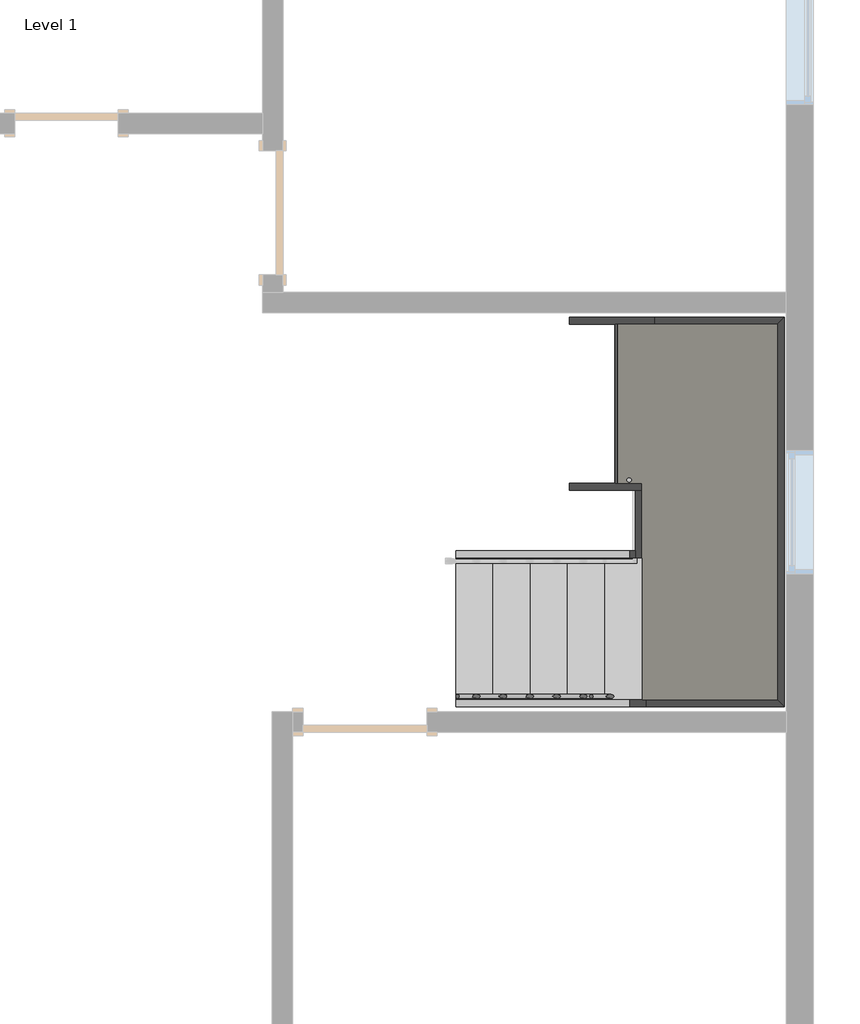
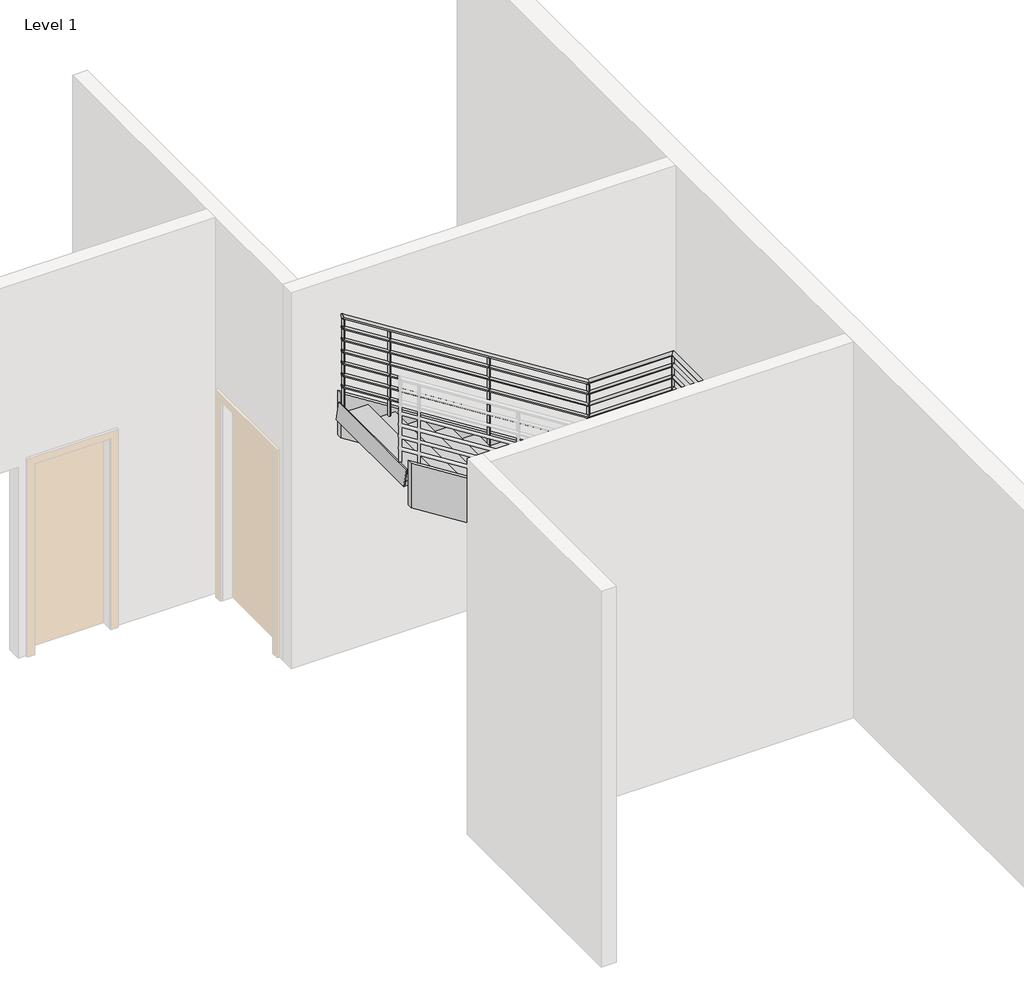
# One storey, part 3 of 3: 8 members, 2 stair flights, 1 railing, 1 slab.
"""IFC4 building model written with IfcOpenShell, lengths in millimetres."""

from ifc_helpers import new_model, si_unit, point, frame, frame_2d, origin, place, context, project, spatial, polyline, circle_curve, ellipse_curve, trimmed, segment, composite_curve, outline, extrude, faceted_brep, transform, mapped, element, save
from ifc_brep_helpers import plane_surface, cylinder_surface, advanced_brep
from components import non_monolithic_landing_709e637c, stair_flight_50mm_tread_25mm_nosing_13mm_riser_430ad9a4, stair_flight_50mm_tread_25mm_nosing_13mm_riser_1a1c1790

model = new_model("IFC4")

# Units and contexts
model_context = context("Model", 3, world=origin())
ifc_project = project(units=[si_unit("LENGTHUNIT", "METRE", prefix="MILLI")], contexts=[model_context])

# Site, building, storey
site = spatial("IfcSite", under=ifc_project)
building = spatial("IfcBuilding", under=site)
storey = spatial("IfcBuildingStorey", under=building, Name="Level 1", Elevation=0.0)

# Members
placement = place(None, origin())
element("IfcMember", 1, ObjectType="Stringer - 50mm Width", at=placement, inside=storey, context=model_context, shape_type="SweptSolid", body=[
    extrude(outline(polyline([(389.0025785, -528.272677), (0.0, -528.272677), (0.0, -395.0139442), (753.6703666, 796.727323), (1226.9472425, 796.727323), (389.0025785, -528.272677)])), frame((0.0, 4121.4539608, 0.0), z_axis=(0.0, 1.0, 0.0), x_axis=(0.0, 0.0, 1.0)), (0.0, 0.0, 1.0), 50.0),
])
element("IfcMember", 2, ObjectType="Stringer - 50mm Width", at=placement, inside=storey, context=model_context, shape_type="SweptSolid", body=[
    extrude(outline(polyline([(389.0025785, -528.272677), (0.0, -528.272677), (0.0, -395.0139442), (864.7850313, 972.4273866), (1264.7850313, 856.5583266), (389.0025785, -528.272677)])), frame((0.0, 3021.4281795, 0.0), z_axis=(0.0, 1.0, 0.0), x_axis=(0.0, 0.0, 1.0)), (0.0, 0.0, 1.0), 50.0),
])
element("IfcMember", 3, ObjectType="Stringer - 50mm Width", at=placement, inside=storey, context=model_context, shape_type="SweptSolid", body=[
    extrude(outline(polyline([(864.7850313, 846.727323), (1334.7593813, 846.727323), (2823.7851872, -1507.7947325), (2350.5083113, -1507.7947325), (864.7850313, 841.5052039), (864.7850313, 846.727323)])), frame((0.0, 4618.9227481, 0.0), z_axis=(0.0, 1.0, 0.0), x_axis=(0.0, 0.0, 1.0)), (0.0, 0.0, 1.0), 50.0),
])
element("IfcMember", 4, ObjectType="Stringer - 50mm Width", at=placement, inside=storey, context=model_context, shape_type="SweptSolid", body=[
    extrude(outline(polyline([(864.7850313, 841.5052039), (1264.7850313, 957.3742639), (2823.7851872, -1507.7947325), (2350.5083113, -1507.7947325), (864.7850313, 841.5052039)])), frame((0.0, 5845.1517528, 0.0), z_axis=(0.0, 1.0, 0.0), x_axis=(0.0, 0.0, 1.0)), (0.0, 0.0, 1.0), 50.0),
])
element("IfcMember", 5, ObjectType="Stringer - 50mm Width", at=placement, inside=storey, context=model_context, shape_type="SweptSolid", body=[
    extrude(outline(polyline([(796.727323, 4618.9227481), (846.727323, 4618.9227481), (846.727323, 4121.4539608), (796.727323, 4121.4539608), (796.727323, 4618.9227481)])), frame((0.0, 0.0, 864.7850313), z_axis=(0.0, 0.0, 1.0), x_axis=(1.0, 0.0, 0.0)), (0.0, 0.0, 1.0), 400.0),
])
element("IfcMember", 6, ObjectType="Stringer - 50mm Width", at=placement, inside=storey, context=model_context, shape_type="Brep", body=[
    faceted_brep([(856.5583266, 3071.4281795, 1264.7850313), (856.5583266, 3021.4281795, 1264.7850313), (1896.7531043, 3021.4281795, 1264.7850313), (1846.7531043, 3071.4281795, 1264.7850313), (972.4273866, 3071.4281795, 864.7850313), (1846.7531043, 3071.4281795, 864.7850313), (972.4273866, 3021.4281795, 864.7850313), (1896.7531043, 3021.4281795, 864.7850313)], [[[0, 1, 2, 3]], [[4, 0, 3, 5]], [[6, 4, 5, 7]], [[1, 6, 7, 2]], [[1, 0, 4, 6]], [[2, 7, 5, 3]]]),
])
element("IfcMember", 7, ObjectType="Stringer - 50mm Width", at=placement, inside=storey, context=model_context, shape_type="SweptSolid", body=[
    extrude(outline(polyline([(1896.7531043, 3021.4281795), (1846.7531043, 3071.4281795), (1846.7531043, 5845.1517528), (1896.7531043, 5895.1517528), (1896.7531043, 3021.4281795)])), frame((0.0, 0.0, 864.7850313), z_axis=(0.0, 0.0, 1.0), x_axis=(1.0, 0.0, 0.0)), (0.0, 0.0, 1.0), 400.0),
])
element("IfcMember", 8, ObjectType="Stringer - 50mm Width", at=placement, inside=storey, context=model_context, shape_type="Brep", body=[
    faceted_brep([(1846.7531043, 5845.1517528, 1264.7850313), (1896.7531043, 5895.1517528, 1264.7850313), (957.3742639, 5895.1517528, 1264.7850313), (957.3742639, 5845.1517528, 1264.7850313), (1846.7531043, 5845.1517528, 864.7850313), (841.5052039, 5845.1517528, 864.7850313), (1896.7531043, 5895.1517528, 864.7850313), (841.5052039, 5895.1517528, 864.7850313)], [[[0, 1, 2, 3]], [[4, 0, 3, 5]], [[6, 4, 5, 7]], [[1, 6, 7, 2]], [[1, 0, 4, 6]], [[2, 7, 5, 3]]]),
])

# Railing
element("IfcRailing", 9, ObjectType="900mm Pipe", at=placement, inside=storey, context=model_context, shape_type="SolidModel", body=[
    advanced_brep(
    [(-528.272677, 3076.8281795, 1224.1622432), (-528.272677, 3116.8281795, 1224.1622432), (852.520776, 3076.8281795, 2097.3913043), (852.520776, 3116.8281795, 2097.3913043), (1841.3531043, 3076.8281795, 2097.3913043), (1801.3531043, 3116.8281795, 2097.3913043), (1841.3531043, 5839.7517528, 2097.3913043), (1801.3531043, 5799.7517528, 2097.3913043), (961.4118145, 5839.7517528, 2097.3913043), (961.4118145, 5799.7517528, 2097.3913043), (-1507.7947325, 5839.7517528, 3658.9448519), (-1507.7947325, 5799.7517528, 3658.9448519)],
    [
        (0, 1, ellipse_curve(frame((-528.272677, 3096.8281795, 1224.1622432), z_axis=(-1.0, 0.0, 0.0), x_axis=(0.0, 0.0, -1.0)), 23.6638438, 20.0)),
        (1, 0, ellipse_curve(frame((-528.272677, 3096.8281795, 1224.1622432), z_axis=(-1.0, 0.0, 0.0), x_axis=(0.0, 0.0, -1.0)), 23.6638438, 20.0)),
        (0, 2),
        (2, 3, ellipse_curve(frame((852.520776, 3096.8281795, 2097.3913043), z_axis=(-0.9605132043335073, 0.0, -0.2782344053149755), x_axis=(0.27823440531497556, 0.0, -0.9605132043335073)), 20.822202, 20.0)),
        (3, 1),
        (3, 2, ellipse_curve(frame((852.520776, 3096.8281795, 2097.3913043), z_axis=(-0.9605132043335073, 0.0, -0.2782344053149755), x_axis=(0.27823440531497556, 0.0, -0.9605132043335073)), 20.822202, 20.0)),
        (2, 4),
        (4, 5, ellipse_curve(frame((1821.3531043, 3096.8281795, 2097.3913043), z_axis=(-0.7071067811865501, -0.7071067811865449, 0.0), x_axis=(-0.7071067811865449, 0.7071067811865501, 0.0)), 28.2842712, 20.0)),
        (5, 3),
        (5, 4, ellipse_curve(frame((1821.3531043, 3096.8281795, 2097.3913043), z_axis=(-0.7071067811865501, -0.7071067811865449, 0.0), x_axis=(-0.7071067811865449, 0.7071067811865501, 0.0)), 28.2842712, 20.0)),
        (4, 6),
        (6, 7, ellipse_curve(frame((1821.3531043, 5819.7517528, 2097.3913043), z_axis=(0.7071067811865449, -0.7071067811865501, 0.0), x_axis=(-0.70710678118655, -0.707106781186545, 0.0)), 28.2842712, 20.0)),
        (7, 5),
        (7, 6, ellipse_curve(frame((1821.3531043, 5819.7517528, 2097.3913043), z_axis=(0.7071067811865449, -0.7071067811865501, 0.0), x_axis=(-0.70710678118655, -0.707106781186545, 0.0)), 28.2842712, 20.0)),
        (6, 8),
        (8, 9, ellipse_curve(frame((961.4118145, 5819.7517528, 2097.3913043), z_axis=(0.9605132043335073, 0.0, -0.2782344053149753), x_axis=(0.27823440531497584, 0.0, 0.9605132043335073)), 20.822202, 20.0)),
        (9, 7),
        (9, 8, ellipse_curve(frame((961.4118145, 5819.7517528, 2097.3913043), z_axis=(0.9605132043335073, 0.0, -0.2782344053149753), x_axis=(0.27823440531497584, 0.0, 0.9605132043335073)), 20.822202, 20.0)),
        (10, 11, ellipse_curve(frame((-1507.7947325, 5819.7517528, 3658.9448519), z_axis=(-1.0, 0.0, 0.0), x_axis=(0.0, 0.0, -1.0)), 23.6638438, 20.0)),
        (11, 10, ellipse_curve(frame((-1507.7947325, 5819.7517528, 3658.9448519), z_axis=(-1.0, 0.0, 0.0), x_axis=(0.0, 0.0, -1.0)), 23.6638438, 20.0)),
        (8, 10),
        (11, 9),
    ],
    [
        plane_surface(frame((-528.272677, 3096.8281795, 1247.826087), z_axis=(-1.0, 0.0, 0.0), x_axis=(0.0, 1.0, 0.0))),
        cylinder_surface(frame((-517.5827642, 3096.8281795, 1230.9226623), z_axis=(-0.8451712313980438, 0.0, -0.5344956404098301), x_axis=(0.0, 1.0, 0.0)), 20.0),
        cylinder_surface(frame((846.727323, 3096.8281795, 2097.3913043), z_axis=(-1.0, 0.0, 0.0), x_axis=(0.0, 1.0, 0.0)), 20.0),
        cylinder_surface(frame((1821.3531043, 3096.8281795, 2097.3913043), z_axis=(0.0, -1.0, 0.0), x_axis=(-1.0, 0.0, 0.0)), 20.0),
        cylinder_surface(frame((1821.3531043, 5819.7517528, 2097.3913043), z_axis=(1.0, 0.0, 0.0), x_axis=(0.0, -1.0, 0.0)), 20.0),
        plane_surface(frame((-1507.7947325, 5819.7517528, 3682.6086957), z_axis=(-1.0, 0.0, 0.0), x_axis=(0.0, -1.0, 0.0))),
        cylinder_surface(frame((956.5153547, 5819.7517528, 2100.4878797), z_axis=(0.8451712313980441, 0.0, -0.5344956404098297), x_axis=(0.0, -1.0, 0.0)), 20.0),
    ],
    [
        (0, [[1, 2]]),
        (1, [[-1, 3, 4, 5]]),
        (1, [[-2, -5, 6, -3]]),
        (2, [[-4, 7, 8, 9]]),
        (2, [[-6, -9, 10, -7]]),
        (3, [[-8, 11, 12, 13]]),
        (3, [[-10, -13, 14, -11]]),
        (4, [[-12, 15, 16, 17]]),
        (4, [[-14, -17, 18, -15]]),
        (5, [[19, 20]]),
        (6, [[-16, 21, -20, 22]]),
        (6, [[-18, -22, -19, -21]]),
    ],
),
    advanced_brep(
    [(-528.272677, 3111.8281795, 1105.0782041), (-528.272677, 3081.8281795, 1105.0782041), (851.0724128, 3111.8281795, 1977.3913043), (851.0724128, 3081.8281795, 1977.3913043), (1806.3531043, 3111.8281795, 1977.3913043), (1836.3531043, 3081.8281795, 1977.3913043), (1806.3531043, 5804.7517528, 1977.3913043), (1836.3531043, 5834.7517528, 1977.3913043), (962.8601777, 5804.7517528, 1977.3913043), (962.8601777, 5834.7517528, 1977.3913043), (-1507.7947325, 5804.7517528, 3539.8608128), (-1507.7947325, 5834.7517528, 3539.8608128)],
    [
        (0, 1, ellipse_curve(frame((-528.272677, 3096.8281795, 1105.0782041), z_axis=(-1.0, 0.0, 0.0), x_axis=(0.0, 0.0, -1.0)), 17.7478828, 15.0)),
        (1, 0, ellipse_curve(frame((-528.272677, 3096.8281795, 1105.0782041), z_axis=(-1.0, 0.0, 0.0), x_axis=(0.0, 0.0, -1.0)), 17.7478828, 15.0)),
        (0, 2),
        (2, 3, ellipse_curve(frame((851.0724128, 3096.8281795, 1977.3913043), z_axis=(-0.9605132043335072, 0.0, -0.2782344053149755), x_axis=(0.2782344053149752, 0.0, -0.9605132043335075)), 15.6166515, 15.0)),
        (3, 1),
        (3, 2, ellipse_curve(frame((851.0724128, 3096.8281795, 1977.3913043), z_axis=(-0.9605132043335072, 0.0, -0.2782344053149755), x_axis=(0.2782344053149752, 0.0, -0.9605132043335075)), 15.6166515, 15.0)),
        (2, 4),
        (4, 5, ellipse_curve(frame((1821.3531043, 3096.8281795, 1977.3913043), z_axis=(-0.7071067811865501, -0.7071067811865449, 0.0), x_axis=(-0.7071067811865449, 0.7071067811865501, 0.0)), 21.2132034, 15.0)),
        (5, 3),
        (5, 4, ellipse_curve(frame((1821.3531043, 3096.8281795, 1977.3913043), z_axis=(-0.7071067811865501, -0.7071067811865449, 0.0), x_axis=(-0.7071067811865449, 0.7071067811865501, 0.0)), 21.2132034, 15.0)),
        (4, 6),
        (6, 7, ellipse_curve(frame((1821.3531043, 5819.7517528, 1977.3913043), z_axis=(0.7071067811865449, -0.7071067811865501, 0.0), x_axis=(-0.70710678118655, -0.707106781186545, 0.0)), 21.2132034, 15.0)),
        (7, 5),
        (7, 6, ellipse_curve(frame((1821.3531043, 5819.7517528, 1977.3913043), z_axis=(0.7071067811865449, -0.7071067811865501, 0.0), x_axis=(-0.70710678118655, -0.707106781186545, 0.0)), 21.2132034, 15.0)),
        (6, 8),
        (8, 9, ellipse_curve(frame((962.8601777, 5819.7517528, 1977.3913043), z_axis=(0.9605132043335073, 0.0, -0.27823440531497523), x_axis=(0.2782344053149759, 0.0, 0.9605132043335072)), 15.6166515, 15.0)),
        (9, 7),
        (9, 8, ellipse_curve(frame((962.8601777, 5819.7517528, 1977.3913043), z_axis=(0.9605132043335073, 0.0, -0.27823440531497523), x_axis=(0.2782344053149759, 0.0, 0.9605132043335072)), 15.6166515, 15.0)),
        (10, 11, ellipse_curve(frame((-1507.7947325, 5819.7517528, 3539.8608128), z_axis=(-1.0, 0.0, 0.0), x_axis=(0.0, 0.0, -1.0)), 17.7478828, 15.0)),
        (11, 10, ellipse_curve(frame((-1507.7947325, 5819.7517528, 3539.8608128), z_axis=(-1.0, 0.0, 0.0), x_axis=(0.0, 0.0, -1.0)), 17.7478828, 15.0)),
        (8, 10),
        (11, 9),
    ],
    [
        plane_surface(frame((-528.272677, 3096.8281795, 1122.826087), z_axis=(-1.0, 0.0, 0.0), x_axis=(0.0, 1.0, 0.0))),
        cylinder_surface(frame((-520.2552424, 3096.8281795, 1110.1485185), z_axis=(-0.8451712313980437, 0.0, -0.5344956404098301), x_axis=(0.0, -1.0, 0.0)), 15.0),
        cylinder_surface(frame((846.727323, 3096.8281795, 1977.3913043), z_axis=(-1.0, 0.0, 0.0), x_axis=(0.0, -1.0, 0.0)), 15.0),
        cylinder_surface(frame((1821.3531043, 3096.8281795, 1977.3913043), z_axis=(0.0, -1.0, 0.0), x_axis=(1.0, 0.0, 0.0)), 15.0),
        cylinder_surface(frame((1821.3531043, 5819.7517528, 1977.3913043), z_axis=(1.0, 0.0, 0.0), x_axis=(0.0, 1.0, 0.0)), 15.0),
        plane_surface(frame((-1507.7947325, 5819.7517528, 3557.6086957), z_axis=(-1.0, 0.0, 0.0), x_axis=(0.0, -1.0, 0.0))),
        cylinder_surface(frame((959.1878329, 5819.7517528, 1979.7137359), z_axis=(0.8451712313980441, 0.0, -0.5344956404098296), x_axis=(0.0, 1.0, 0.0)), 15.0),
    ],
    [
        (0, [[1, 2]]),
        (1, [[-1, 3, 4, 5]]),
        (1, [[-2, -5, 6, -3]]),
        (2, [[-4, 7, 8, 9]]),
        (2, [[-6, -9, 10, -7]]),
        (3, [[-8, 11, 12, 13]]),
        (3, [[-10, -13, 14, -11]]),
        (4, [[-12, 15, 16, 17]]),
        (4, [[-14, -17, 18, -15]]),
        (5, [[19, 20]]),
        (6, [[-16, 21, -20, 22]]),
        (6, [[-18, -22, -19, -21]]),
    ],
),
    advanced_brep(
    [(-528.272677, 3111.8281795, 980.0782041), (-528.272677, 3081.8281795, 980.0782041), (851.0724128, 3111.8281795, 1852.3913043), (851.0724128, 3081.8281795, 1852.3913043), (1806.3531043, 3111.8281795, 1852.3913043), (1836.3531043, 3081.8281795, 1852.3913043), (1806.3531043, 5804.7517528, 1852.3913043), (1836.3531043, 5834.7517528, 1852.3913043), (962.8601777, 5804.7517528, 1852.3913043), (962.8601777, 5834.7517528, 1852.3913043), (-1507.7947325, 5804.7517528, 3414.8608128), (-1507.7947325, 5834.7517528, 3414.8608128)],
    [
        (0, 1, ellipse_curve(frame((-528.272677, 3096.8281795, 980.0782041), z_axis=(-1.0, 0.0, 0.0), x_axis=(0.0, 0.0, -1.0)), 17.7478828, 15.0)),
        (1, 0, ellipse_curve(frame((-528.272677, 3096.8281795, 980.0782041), z_axis=(-1.0, 0.0, 0.0), x_axis=(0.0, 0.0, -1.0)), 17.7478828, 15.0)),
        (0, 2),
        (2, 3, ellipse_curve(frame((851.0724128, 3096.8281795, 1852.3913043), z_axis=(-0.9605132043335072, 0.0, -0.2782344053149755), x_axis=(0.2782344053149752, 0.0, -0.9605132043335075)), 15.6166515, 15.0)),
        (3, 1),
        (3, 2, ellipse_curve(frame((851.0724128, 3096.8281795, 1852.3913043), z_axis=(-0.9605132043335072, 0.0, -0.2782344053149755), x_axis=(0.2782344053149752, 0.0, -0.9605132043335075)), 15.6166515, 15.0)),
        (2, 4),
        (4, 5, ellipse_curve(frame((1821.3531043, 3096.8281795, 1852.3913043), z_axis=(-0.7071067811865501, -0.7071067811865449, 0.0), x_axis=(-0.7071067811865449, 0.7071067811865501, 0.0)), 21.2132034, 15.0)),
        (5, 3),
        (5, 4, ellipse_curve(frame((1821.3531043, 3096.8281795, 1852.3913043), z_axis=(-0.7071067811865501, -0.7071067811865449, 0.0), x_axis=(-0.7071067811865449, 0.7071067811865501, 0.0)), 21.2132034, 15.0)),
        (4, 6),
        (6, 7, ellipse_curve(frame((1821.3531043, 5819.7517528, 1852.3913043), z_axis=(0.7071067811865449, -0.7071067811865501, 0.0), x_axis=(-0.70710678118655, -0.707106781186545, 0.0)), 21.2132034, 15.0)),
        (7, 5),
        (7, 6, ellipse_curve(frame((1821.3531043, 5819.7517528, 1852.3913043), z_axis=(0.7071067811865449, -0.7071067811865501, 0.0), x_axis=(-0.70710678118655, -0.707106781186545, 0.0)), 21.2132034, 15.0)),
        (6, 8),
        (8, 9, ellipse_curve(frame((962.8601777, 5819.7517528, 1852.3913043), z_axis=(0.9605132043335073, 0.0, -0.2782344053149753), x_axis=(0.27823440531497584, 0.0, 0.9605132043335073)), 15.6166515, 15.0)),
        (9, 7),
        (9, 8, ellipse_curve(frame((962.8601777, 5819.7517528, 1852.3913043), z_axis=(0.9605132043335073, 0.0, -0.2782344053149753), x_axis=(0.27823440531497584, 0.0, 0.9605132043335073)), 15.6166515, 15.0)),
        (10, 11, ellipse_curve(frame((-1507.7947325, 5819.7517528, 3414.8608128), z_axis=(-1.0, 0.0, 0.0), x_axis=(0.0, 0.0, -1.0)), 17.7478828, 15.0)),
        (11, 10, ellipse_curve(frame((-1507.7947325, 5819.7517528, 3414.8608128), z_axis=(-1.0, 0.0, 0.0), x_axis=(0.0, 0.0, -1.0)), 17.7478828, 15.0)),
        (8, 10),
        (11, 9),
    ],
    [
        plane_surface(frame((-528.272677, 3096.8281795, 997.826087), z_axis=(-1.0, 0.0, 0.0), x_axis=(0.0, 1.0, 0.0))),
        cylinder_surface(frame((-520.2552424, 3096.8281795, 985.1485185), z_axis=(-0.8451712313980437, 0.0, -0.5344956404098301), x_axis=(0.0, -1.0, 0.0)), 15.0),
        cylinder_surface(frame((846.727323, 3096.8281795, 1852.3913043), z_axis=(-1.0, 0.0, 0.0), x_axis=(0.0, -1.0, 0.0)), 15.0),
        cylinder_surface(frame((1821.3531043, 3096.8281795, 1852.3913043), z_axis=(0.0, -1.0, 0.0), x_axis=(1.0, 0.0, 0.0)), 15.0),
        cylinder_surface(frame((1821.3531043, 5819.7517528, 1852.3913043), z_axis=(1.0, 0.0, 0.0), x_axis=(0.0, 1.0, 0.0)), 15.0),
        plane_surface(frame((-1507.7947325, 5819.7517528, 3432.6086957), z_axis=(-1.0, 0.0, 0.0), x_axis=(0.0, -1.0, 0.0))),
        cylinder_surface(frame((959.1878329, 5819.7517528, 1854.7137359), z_axis=(0.8451712313980441, 0.0, -0.5344956404098297), x_axis=(0.0, 1.0, 0.0)), 15.0),
    ],
    [
        (0, [[1, 2]]),
        (1, [[-1, 3, 4, 5]]),
        (1, [[-2, -5, 6, -3]]),
        (2, [[-4, 7, 8, 9]]),
        (2, [[-6, -9, 10, -7]]),
        (3, [[-8, 11, 12, 13]]),
        (3, [[-10, -13, 14, -11]]),
        (4, [[-12, 15, 16, 17]]),
        (4, [[-14, -17, 18, -15]]),
        (5, [[19, 20]]),
        (6, [[-16, 21, -20, 22]]),
        (6, [[-18, -22, -19, -21]]),
    ],
),
    advanced_brep(
    [(-528.272677, 3111.8281795, 855.0782041), (-528.272677, 3081.8281795, 855.0782041), (851.0724128, 3111.8281795, 1727.3913043), (851.0724128, 3081.8281795, 1727.3913043), (1806.3531043, 3111.8281795, 1727.3913043), (1836.3531043, 3081.8281795, 1727.3913043), (1806.3531043, 5804.7517528, 1727.3913043), (1836.3531043, 5834.7517528, 1727.3913043), (962.8601777, 5804.7517528, 1727.3913043), (962.8601777, 5834.7517528, 1727.3913043), (-1507.7947325, 5804.7517528, 3289.8608128), (-1507.7947325, 5834.7517528, 3289.8608128)],
    [
        (0, 1, ellipse_curve(frame((-528.272677, 3096.8281795, 855.0782041), z_axis=(-1.0, 0.0, 0.0), x_axis=(0.0, 0.0, -1.0)), 17.7478828, 15.0)),
        (1, 0, ellipse_curve(frame((-528.272677, 3096.8281795, 855.0782041), z_axis=(-1.0, 0.0, 0.0), x_axis=(0.0, 0.0, -1.0)), 17.7478828, 15.0)),
        (0, 2),
        (2, 3, ellipse_curve(frame((851.0724128, 3096.8281795, 1727.3913043), z_axis=(-0.9605132043335072, 0.0, -0.2782344053149755), x_axis=(0.2782344053149752, 0.0, -0.9605132043335075)), 15.6166515, 15.0)),
        (3, 1),
        (3, 2, ellipse_curve(frame((851.0724128, 3096.8281795, 1727.3913043), z_axis=(-0.9605132043335072, 0.0, -0.2782344053149755), x_axis=(0.2782344053149752, 0.0, -0.9605132043335075)), 15.6166515, 15.0)),
        (2, 4),
        (4, 5, ellipse_curve(frame((1821.3531043, 3096.8281795, 1727.3913043), z_axis=(-0.7071067811865501, -0.7071067811865449, 0.0), x_axis=(-0.7071067811865449, 0.7071067811865501, 0.0)), 21.2132034, 15.0)),
        (5, 3),
        (5, 4, ellipse_curve(frame((1821.3531043, 3096.8281795, 1727.3913043), z_axis=(-0.7071067811865501, -0.7071067811865449, 0.0), x_axis=(-0.7071067811865449, 0.7071067811865501, 0.0)), 21.2132034, 15.0)),
        (4, 6),
        (6, 7, ellipse_curve(frame((1821.3531043, 5819.7517528, 1727.3913043), z_axis=(0.7071067811865449, -0.7071067811865501, 0.0), x_axis=(-0.70710678118655, -0.707106781186545, 0.0)), 21.2132034, 15.0)),
        (7, 5),
        (7, 6, ellipse_curve(frame((1821.3531043, 5819.7517528, 1727.3913043), z_axis=(0.7071067811865449, -0.7071067811865501, 0.0), x_axis=(-0.70710678118655, -0.707106781186545, 0.0)), 21.2132034, 15.0)),
        (6, 8),
        (8, 9, ellipse_curve(frame((962.8601777, 5819.7517528, 1727.3913043), z_axis=(0.9605132043335073, 0.0, -0.2782344053149753), x_axis=(0.27823440531497584, 0.0, 0.9605132043335073)), 15.6166515, 15.0)),
        (9, 7),
        (9, 8, ellipse_curve(frame((962.8601777, 5819.7517528, 1727.3913043), z_axis=(0.9605132043335073, 0.0, -0.2782344053149753), x_axis=(0.27823440531497584, 0.0, 0.9605132043335073)), 15.6166515, 15.0)),
        (10, 11, ellipse_curve(frame((-1507.7947325, 5819.7517528, 3289.8608128), z_axis=(-1.0, 0.0, 0.0), x_axis=(0.0, 0.0, -1.0)), 17.7478828, 15.0)),
        (11, 10, ellipse_curve(frame((-1507.7947325, 5819.7517528, 3289.8608128), z_axis=(-1.0, 0.0, 0.0), x_axis=(0.0, 0.0, -1.0)), 17.7478828, 15.0)),
        (8, 10),
        (11, 9),
    ],
    [
        plane_surface(frame((-528.272677, 3096.8281795, 872.826087), z_axis=(-1.0, 0.0, 0.0), x_axis=(0.0, 1.0, 0.0))),
        cylinder_surface(frame((-520.2552424, 3096.8281795, 860.1485185), z_axis=(-0.8451712313980437, 0.0, -0.5344956404098301), x_axis=(0.0, -1.0, 0.0)), 15.0),
        cylinder_surface(frame((846.727323, 3096.8281795, 1727.3913043), z_axis=(-1.0, 0.0, 0.0), x_axis=(0.0, -1.0, 0.0)), 15.0),
        cylinder_surface(frame((1821.3531043, 3096.8281795, 1727.3913043), z_axis=(0.0, -1.0, 0.0), x_axis=(1.0, 0.0, 0.0)), 15.0),
        cylinder_surface(frame((1821.3531043, 5819.7517528, 1727.3913043), z_axis=(1.0, 0.0, 0.0), x_axis=(0.0, 1.0, 0.0)), 15.0),
        plane_surface(frame((-1507.7947325, 5819.7517528, 3307.6086957), z_axis=(-1.0, 0.0, 0.0), x_axis=(0.0, -1.0, 0.0))),
        cylinder_surface(frame((959.1878329, 5819.7517528, 1729.7137359), z_axis=(0.8451712313980441, 0.0, -0.5344956404098297), x_axis=(0.0, 1.0, 0.0)), 15.0),
    ],
    [
        (0, [[1, 2]]),
        (1, [[-1, 3, 4, 5]]),
        (1, [[-2, -5, 6, -3]]),
        (2, [[-4, 7, 8, 9]]),
        (2, [[-6, -9, 10, -7]]),
        (3, [[-8, 11, 12, 13]]),
        (3, [[-10, -13, 14, -11]]),
        (4, [[-12, 15, 16, 17]]),
        (4, [[-14, -17, 18, -15]]),
        (5, [[19, 20]]),
        (6, [[-16, 21, -20, 22]]),
        (6, [[-18, -22, -19, -21]]),
    ],
),
    advanced_brep(
    [(-528.272677, 3111.8281795, 730.0782041), (-528.272677, 3081.8281795, 730.0782041), (851.0724128, 3111.8281795, 1602.3913043), (851.0724128, 3081.8281795, 1602.3913043), (1806.3531043, 3111.8281795, 1602.3913043), (1836.3531043, 3081.8281795, 1602.3913043), (1806.3531043, 5804.7517528, 1602.3913043), (1836.3531043, 5834.7517528, 1602.3913043), (962.8601777, 5804.7517528, 1602.3913043), (962.8601777, 5834.7517528, 1602.3913043), (-1507.7947325, 5804.7517528, 3164.8608128), (-1507.7947325, 5834.7517528, 3164.8608128)],
    [
        (0, 1, ellipse_curve(frame((-528.272677, 3096.8281795, 730.0782041), z_axis=(-1.0, 0.0, 0.0), x_axis=(0.0, 0.0, -1.0)), 17.7478828, 15.0)),
        (1, 0, ellipse_curve(frame((-528.272677, 3096.8281795, 730.0782041), z_axis=(-1.0, 0.0, 0.0), x_axis=(0.0, 0.0, -1.0)), 17.7478828, 15.0)),
        (0, 2),
        (2, 3, ellipse_curve(frame((851.0724128, 3096.8281795, 1602.3913043), z_axis=(-0.9605132043335072, 0.0, -0.2782344053149755), x_axis=(0.2782344053149752, 0.0, -0.9605132043335075)), 15.6166515, 15.0)),
        (3, 1),
        (3, 2, ellipse_curve(frame((851.0724128, 3096.8281795, 1602.3913043), z_axis=(-0.9605132043335072, 0.0, -0.2782344053149755), x_axis=(0.2782344053149752, 0.0, -0.9605132043335075)), 15.6166515, 15.0)),
        (2, 4),
        (4, 5, ellipse_curve(frame((1821.3531043, 3096.8281795, 1602.3913043), z_axis=(-0.7071067811865501, -0.7071067811865449, 0.0), x_axis=(-0.7071067811865449, 0.7071067811865501, 0.0)), 21.2132034, 15.0)),
        (5, 3),
        (5, 4, ellipse_curve(frame((1821.3531043, 3096.8281795, 1602.3913043), z_axis=(-0.7071067811865501, -0.7071067811865449, 0.0), x_axis=(-0.7071067811865449, 0.7071067811865501, 0.0)), 21.2132034, 15.0)),
        (4, 6),
        (6, 7, ellipse_curve(frame((1821.3531043, 5819.7517528, 1602.3913043), z_axis=(0.7071067811865449, -0.7071067811865501, 0.0), x_axis=(-0.70710678118655, -0.707106781186545, 0.0)), 21.2132034, 15.0)),
        (7, 5),
        (7, 6, ellipse_curve(frame((1821.3531043, 5819.7517528, 1602.3913043), z_axis=(0.7071067811865449, -0.7071067811865501, 0.0), x_axis=(-0.70710678118655, -0.707106781186545, 0.0)), 21.2132034, 15.0)),
        (6, 8),
        (8, 9, ellipse_curve(frame((962.8601777, 5819.7517528, 1602.3913043), z_axis=(0.9605132043335073, 0.0, -0.2782344053149753), x_axis=(0.27823440531497584, 0.0, 0.9605132043335073)), 15.6166515, 15.0)),
        (9, 7),
        (9, 8, ellipse_curve(frame((962.8601777, 5819.7517528, 1602.3913043), z_axis=(0.9605132043335073, 0.0, -0.2782344053149753), x_axis=(0.27823440531497584, 0.0, 0.9605132043335073)), 15.6166515, 15.0)),
        (10, 11, ellipse_curve(frame((-1507.7947325, 5819.7517528, 3164.8608128), z_axis=(-1.0, 0.0, 0.0), x_axis=(0.0, 0.0, -1.0)), 17.7478828, 15.0)),
        (11, 10, ellipse_curve(frame((-1507.7947325, 5819.7517528, 3164.8608128), z_axis=(-1.0, 0.0, 0.0), x_axis=(0.0, 0.0, -1.0)), 17.7478828, 15.0)),
        (8, 10),
        (11, 9),
    ],
    [
        plane_surface(frame((-528.272677, 3096.8281795, 747.826087), z_axis=(-1.0, 0.0, 0.0), x_axis=(0.0, 1.0, 0.0))),
        cylinder_surface(frame((-520.2552424, 3096.8281795, 735.1485185), z_axis=(-0.8451712313980437, 0.0, -0.5344956404098301), x_axis=(0.0, -1.0, 0.0)), 15.0),
        cylinder_surface(frame((846.727323, 3096.8281795, 1602.3913043), z_axis=(-1.0, 0.0, 0.0), x_axis=(0.0, -1.0, 0.0)), 15.0),
        cylinder_surface(frame((1821.3531043, 3096.8281795, 1602.3913043), z_axis=(0.0, -1.0, 0.0), x_axis=(1.0, 0.0, 0.0)), 15.0),
        cylinder_surface(frame((1821.3531043, 5819.7517528, 1602.3913043), z_axis=(1.0, 0.0, 0.0), x_axis=(0.0, 1.0, 0.0)), 15.0),
        plane_surface(frame((-1507.7947325, 5819.7517528, 3182.6086957), z_axis=(-1.0, 0.0, 0.0), x_axis=(0.0, -1.0, 0.0))),
        cylinder_surface(frame((959.1878329, 5819.7517528, 1604.7137359), z_axis=(0.8451712313980441, 0.0, -0.5344956404098297), x_axis=(0.0, 1.0, 0.0)), 15.0),
    ],
    [
        (0, [[1, 2]]),
        (1, [[-1, 3, 4, 5]]),
        (1, [[-2, -5, 6, -3]]),
        (2, [[-4, 7, 8, 9]]),
        (2, [[-6, -9, 10, -7]]),
        (3, [[-8, 11, 12, 13]]),
        (3, [[-10, -13, 14, -11]]),
        (4, [[-12, 15, 16, 17]]),
        (4, [[-14, -17, 18, -15]]),
        (5, [[19, 20]]),
        (6, [[-16, 21, -20, 22]]),
        (6, [[-18, -22, -19, -21]]),
    ],
),
    advanced_brep(
    [(-528.272677, 3111.8281795, 605.0782041), (-528.272677, 3081.8281795, 605.0782041), (851.0724128, 3111.8281795, 1477.3913043), (851.0724128, 3081.8281795, 1477.3913043), (1806.3531043, 3111.8281795, 1477.3913043), (1836.3531043, 3081.8281795, 1477.3913043), (1806.3531043, 5804.7517528, 1477.3913043), (1836.3531043, 5834.7517528, 1477.3913043), (962.8601777, 5804.7517528, 1477.3913043), (962.8601777, 5834.7517528, 1477.3913043), (-1507.7947325, 5804.7517528, 3039.8608128), (-1507.7947325, 5834.7517528, 3039.8608128)],
    [
        (0, 1, ellipse_curve(frame((-528.272677, 3096.8281795, 605.0782041), z_axis=(-1.0, 0.0, 0.0), x_axis=(0.0, 0.0, -1.0)), 17.7478828, 15.0)),
        (1, 0, ellipse_curve(frame((-528.272677, 3096.8281795, 605.0782041), z_axis=(-1.0, 0.0, 0.0), x_axis=(0.0, 0.0, -1.0)), 17.7478828, 15.0)),
        (0, 2),
        (2, 3, ellipse_curve(frame((851.0724128, 3096.8281795, 1477.3913043), z_axis=(-0.9605132043335072, 0.0, -0.2782344053149755), x_axis=(0.2782344053149752, 0.0, -0.9605132043335075)), 15.6166515, 15.0)),
        (3, 1),
        (3, 2, ellipse_curve(frame((851.0724128, 3096.8281795, 1477.3913043), z_axis=(-0.9605132043335072, 0.0, -0.2782344053149755), x_axis=(0.2782344053149752, 0.0, -0.9605132043335075)), 15.6166515, 15.0)),
        (2, 4),
        (4, 5, ellipse_curve(frame((1821.3531043, 3096.8281795, 1477.3913043), z_axis=(-0.7071067811865501, -0.7071067811865449, 0.0), x_axis=(-0.7071067811865449, 0.7071067811865501, 0.0)), 21.2132034, 15.0)),
        (5, 3),
        (5, 4, ellipse_curve(frame((1821.3531043, 3096.8281795, 1477.3913043), z_axis=(-0.7071067811865501, -0.7071067811865449, 0.0), x_axis=(-0.7071067811865449, 0.7071067811865501, 0.0)), 21.2132034, 15.0)),
        (4, 6),
        (6, 7, ellipse_curve(frame((1821.3531043, 5819.7517528, 1477.3913043), z_axis=(0.7071067811865449, -0.7071067811865501, 0.0), x_axis=(-0.70710678118655, -0.707106781186545, 0.0)), 21.2132034, 15.0)),
        (7, 5),
        (7, 6, ellipse_curve(frame((1821.3531043, 5819.7517528, 1477.3913043), z_axis=(0.7071067811865449, -0.7071067811865501, 0.0), x_axis=(-0.70710678118655, -0.707106781186545, 0.0)), 21.2132034, 15.0)),
        (6, 8),
        (8, 9, ellipse_curve(frame((962.8601777, 5819.7517528, 1477.3913043), z_axis=(0.9605132043335073, 0.0, -0.27823440531497523), x_axis=(0.2782344053149759, 0.0, 0.9605132043335072)), 15.6166515, 15.0)),
        (9, 7),
        (9, 8, ellipse_curve(frame((962.8601777, 5819.7517528, 1477.3913043), z_axis=(0.9605132043335073, 0.0, -0.27823440531497523), x_axis=(0.2782344053149759, 0.0, 0.9605132043335072)), 15.6166515, 15.0)),
        (10, 11, ellipse_curve(frame((-1507.7947325, 5819.7517528, 3039.8608128), z_axis=(-1.0, 0.0, 0.0), x_axis=(0.0, 0.0, -1.0)), 17.7478828, 15.0)),
        (11, 10, ellipse_curve(frame((-1507.7947325, 5819.7517528, 3039.8608128), z_axis=(-1.0, 0.0, 0.0), x_axis=(0.0, 0.0, -1.0)), 17.7478828, 15.0)),
        (8, 10),
        (11, 9),
    ],
    [
        plane_surface(frame((-528.272677, 3096.8281795, 622.826087), z_axis=(-1.0, 0.0, 0.0), x_axis=(0.0, 1.0, 0.0))),
        cylinder_surface(frame((-520.2552424, 3096.8281795, 610.1485185), z_axis=(-0.8451712313980437, 0.0, -0.5344956404098301), x_axis=(0.0, -1.0, 0.0)), 15.0),
        cylinder_surface(frame((846.727323, 3096.8281795, 1477.3913043), z_axis=(-1.0, 0.0, 0.0), x_axis=(0.0, -1.0, 0.0)), 15.0),
        cylinder_surface(frame((1821.3531043, 3096.8281795, 1477.3913043), z_axis=(0.0, -1.0, 0.0), x_axis=(1.0, 0.0, 0.0)), 15.0),
        cylinder_surface(frame((1821.3531043, 5819.7517528, 1477.3913043), z_axis=(1.0, 0.0, 0.0), x_axis=(0.0, 1.0, 0.0)), 15.0),
        plane_surface(frame((-1507.7947325, 5819.7517528, 3057.6086957), z_axis=(-1.0, 0.0, 0.0), x_axis=(0.0, -1.0, 0.0))),
        cylinder_surface(frame((959.1878329, 5819.7517528, 1479.7137359), z_axis=(0.8451712313980441, 0.0, -0.5344956404098296), x_axis=(0.0, 1.0, 0.0)), 15.0),
    ],
    [
        (0, [[1, 2]]),
        (1, [[-1, 3, 4, 5]]),
        (1, [[-2, -5, 6, -3]]),
        (2, [[-4, 7, 8, 9]]),
        (2, [[-6, -9, 10, -7]]),
        (3, [[-8, 11, 12, 13]]),
        (3, [[-10, -13, 14, -11]]),
        (4, [[-12, 15, 16, 17]]),
        (4, [[-14, -17, 18, -15]]),
        (5, [[19, 20]]),
        (6, [[-16, 21, -20, 22]]),
        (6, [[-18, -22, -19, -21]]),
    ],
),
    advanced_brep(
    [(-528.272677, 3111.8281795, 480.0782041), (-528.272677, 3081.8281795, 480.0782041), (851.0724128, 3111.8281795, 1352.3913043), (851.0724128, 3081.8281795, 1352.3913043), (1806.3531043, 3111.8281795, 1352.3913043), (1836.3531043, 3081.8281795, 1352.3913043), (1806.3531043, 5804.7517528, 1352.3913043), (1836.3531043, 5834.7517528, 1352.3913043), (962.8601777, 5804.7517528, 1352.3913043), (962.8601777, 5834.7517528, 1352.3913043), (-1507.7947325, 5804.7517528, 2914.8608128), (-1507.7947325, 5834.7517528, 2914.8608128)],
    [
        (0, 1, ellipse_curve(frame((-528.272677, 3096.8281795, 480.0782041), z_axis=(-1.0, 0.0, 0.0), x_axis=(0.0, 0.0, -1.0)), 17.7478828, 15.0)),
        (1, 0, ellipse_curve(frame((-528.272677, 3096.8281795, 480.0782041), z_axis=(-1.0, 0.0, 0.0), x_axis=(0.0, 0.0, -1.0)), 17.7478828, 15.0)),
        (0, 2),
        (2, 3, ellipse_curve(frame((851.0724128, 3096.8281795, 1352.3913043), z_axis=(-0.9605132043335072, 0.0, -0.2782344053149755), x_axis=(0.2782344053149752, 0.0, -0.9605132043335075)), 15.6166515, 15.0)),
        (3, 1),
        (3, 2, ellipse_curve(frame((851.0724128, 3096.8281795, 1352.3913043), z_axis=(-0.9605132043335072, 0.0, -0.2782344053149755), x_axis=(0.2782344053149752, 0.0, -0.9605132043335075)), 15.6166515, 15.0)),
        (2, 4),
        (4, 5, ellipse_curve(frame((1821.3531043, 3096.8281795, 1352.3913043), z_axis=(-0.7071067811865501, -0.7071067811865449, 0.0), x_axis=(-0.7071067811865449, 0.7071067811865501, 0.0)), 21.2132034, 15.0)),
        (5, 3),
        (5, 4, ellipse_curve(frame((1821.3531043, 3096.8281795, 1352.3913043), z_axis=(-0.7071067811865501, -0.7071067811865449, 0.0), x_axis=(-0.7071067811865449, 0.7071067811865501, 0.0)), 21.2132034, 15.0)),
        (4, 6),
        (6, 7, ellipse_curve(frame((1821.3531043, 5819.7517528, 1352.3913043), z_axis=(0.7071067811865449, -0.7071067811865501, 0.0), x_axis=(-0.70710678118655, -0.707106781186545, 0.0)), 21.2132034, 15.0)),
        (7, 5),
        (7, 6, ellipse_curve(frame((1821.3531043, 5819.7517528, 1352.3913043), z_axis=(0.7071067811865449, -0.7071067811865501, 0.0), x_axis=(-0.70710678118655, -0.707106781186545, 0.0)), 21.2132034, 15.0)),
        (6, 8),
        (8, 9, ellipse_curve(frame((962.8601777, 5819.7517528, 1352.3913043), z_axis=(0.9605132043335073, 0.0, -0.2782344053149753), x_axis=(0.27823440531497584, 0.0, 0.9605132043335073)), 15.6166515, 15.0)),
        (9, 7),
        (9, 8, ellipse_curve(frame((962.8601777, 5819.7517528, 1352.3913043), z_axis=(0.9605132043335073, 0.0, -0.2782344053149753), x_axis=(0.27823440531497584, 0.0, 0.9605132043335073)), 15.6166515, 15.0)),
        (10, 11, ellipse_curve(frame((-1507.7947325, 5819.7517528, 2914.8608128), z_axis=(-1.0, 0.0, 0.0), x_axis=(0.0, 0.0, -1.0)), 17.7478828, 15.0)),
        (11, 10, ellipse_curve(frame((-1507.7947325, 5819.7517528, 2914.8608128), z_axis=(-1.0, 0.0, 0.0), x_axis=(0.0, 0.0, -1.0)), 17.7478828, 15.0)),
        (8, 10),
        (11, 9),
    ],
    [
        plane_surface(frame((-528.272677, 3096.8281795, 497.826087), z_axis=(-1.0, 0.0, 0.0), x_axis=(0.0, 1.0, 0.0))),
        cylinder_surface(frame((-520.2552424, 3096.8281795, 485.1485185), z_axis=(-0.8451712313980437, 0.0, -0.5344956404098301), x_axis=(0.0, -1.0, 0.0)), 15.0),
        cylinder_surface(frame((846.727323, 3096.8281795, 1352.3913043), z_axis=(-1.0, 0.0, 0.0), x_axis=(0.0, -1.0, 0.0)), 15.0),
        cylinder_surface(frame((1821.3531043, 3096.8281795, 1352.3913043), z_axis=(0.0, -1.0, 0.0), x_axis=(1.0, 0.0, 0.0)), 15.0),
        cylinder_surface(frame((1821.3531043, 5819.7517528, 1352.3913043), z_axis=(1.0, 0.0, 0.0), x_axis=(0.0, 1.0, 0.0)), 15.0),
        plane_surface(frame((-1507.7947325, 5819.7517528, 2932.6086957), z_axis=(-1.0, 0.0, 0.0), x_axis=(0.0, -1.0, 0.0))),
        cylinder_surface(frame((959.1878329, 5819.7517528, 1354.7137359), z_axis=(0.8451712313980441, 0.0, -0.5344956404098297), x_axis=(0.0, 1.0, 0.0)), 15.0),
    ],
    [
        (0, [[1, 2]]),
        (1, [[-1, 3, 4, 5]]),
        (1, [[-2, -5, 6, -3]]),
        (2, [[-4, 7, 8, 9]]),
        (2, [[-6, -9, 10, -7]]),
        (3, [[-8, 11, 12, 13]]),
        (3, [[-10, -13, 14, -11]]),
        (4, [[-12, 15, 16, 17]]),
        (4, [[-14, -17, 18, -15]]),
        (5, [[19, 20]]),
        (6, [[-16, 21, -20, 22]]),
        (6, [[-18, -22, -19, -21]]),
    ],
),
    advanced_brep(
    [(-1032.7947325, 5832.2517528, 3334.8857511), (-1032.7947325, 5832.2517528, 2434.7826087), (-1032.7947325, 5807.2517528, 2434.7826087), (-1032.7947325, 5807.2517528, 3334.8857511)],
    [
        (0, 1),
        (1, 2, circle_curve(frame((-1032.7947325, 5819.7517528, 2434.7826087), z_axis=(0.0, 0.0, 1.0), x_axis=(0.0, -1.0, 0.0)), 12.5)),
        (2, 3),
        (3, 0, ellipse_curve(frame((-1032.7947325, 5819.7517528, 3334.8857511), z_axis=(-0.5344956404098286, 0.0, -0.8451712313980447), x_axis=(-0.8451712313980447, 0.0, 0.5344956404098286)), 14.7899024, 12.5)),
        (0, 3, ellipse_curve(frame((-1032.7947325, 5819.7517528, 3334.8857511), z_axis=(-0.5344956404098286, 0.0, -0.8451712313980447), x_axis=(-0.8451712313980447, 0.0, 0.5344956404098286)), 14.7899024, 12.5)),
        (2, 1, circle_curve(frame((-1032.7947325, 5819.7517528, 2434.7826087), z_axis=(0.0, 0.0, 1.0), x_axis=(0.0, -1.0, 0.0)), 12.5)),
    ],
    [
        cylinder_surface(frame((-1032.7947325, 5819.7517528, 2334.7826087), z_axis=(0.0, 0.0, 1.0), x_axis=(0.0, -1.0, 0.0)), 12.5),
        plane_surface(frame((-1057.7947325, 5794.7517528, 3350.6960278), z_axis=(0.5344956404098286, 0.0, 0.8451712313980447), x_axis=(0.0, 1.0, 0.0))),
        plane_surface(frame((-1007.7947325, 5794.7517528, 2434.7826087), z_axis=(0.0, 0.0, -1.0), x_axis=(0.0, 1.0, 0.0))),
    ],
    [
        (0, [[1, 2, 3, 4]]),
        (0, [[-1, 5, -3, 6]]),
        (1, [[-4, -5]]),
        (2, [[-2, -6]]),
    ],
),
    advanced_brep(
    [(-32.7947325, 5832.2517528, 2702.474684), (-32.7947325, 5832.2517528, 1739.1304348), (-32.7947325, 5807.2517528, 1739.1304348), (-32.7947325, 5807.2517528, 2702.474684)],
    [
        (0, 1),
        (1, 2, circle_curve(frame((-32.7947325, 5819.7517528, 1739.1304348), z_axis=(0.0, 0.0, 1.0), x_axis=(0.0, -1.0, 0.0)), 12.5)),
        (2, 3),
        (3, 0, ellipse_curve(frame((-32.7947325, 5819.7517528, 2702.474684), z_axis=(-0.5344956404098286, 0.0, -0.8451712313980447), x_axis=(-0.8451712313980447, 0.0, 0.5344956404098286)), 14.7899024, 12.5)),
        (0, 3, ellipse_curve(frame((-32.7947325, 5819.7517528, 2702.474684), z_axis=(-0.5344956404098286, 0.0, -0.8451712313980447), x_axis=(-0.8451712313980447, 0.0, 0.5344956404098286)), 14.7899024, 12.5)),
        (2, 1, circle_curve(frame((-32.7947325, 5819.7517528, 1739.1304348), z_axis=(0.0, 0.0, 1.0), x_axis=(0.0, -1.0, 0.0)), 12.5)),
    ],
    [
        cylinder_surface(frame((-32.7947325, 5819.7517528, 1639.1304348), z_axis=(0.0, 0.0, 1.0), x_axis=(0.0, -1.0, 0.0)), 12.5),
        plane_surface(frame((-57.7947325, 5794.7517528, 2718.2849606), z_axis=(0.5344956404098286, 0.0, 0.8451712313980447), x_axis=(0.0, 1.0, 0.0))),
        plane_surface(frame((-7.7947325, 5794.7517528, 1739.1304348), z_axis=(0.0, 0.0, -1.0), x_axis=(0.0, 1.0, 0.0))),
    ],
    [
        (0, [[1, 2, 3, 4]]),
        (0, [[-1, 5, -3, 6]]),
        (1, [[-4, -5]]),
        (2, [[-2, -6]]),
    ],
),
    extrude(outline(composite_curve([segment(trimmed(circle_curve(frame_2d((1821.3531043, 5096.8281795)), 12.5), [point((1808.8531043, 5096.8281795))], [point((1833.8531043, 5096.8281795))], False, "CARTESIAN"), True, "CONTINUOUS"), segment(trimmed(circle_curve(frame_2d((1821.3531043, 5096.8281795)), 12.5), [point((1833.8531043, 5096.8281795))], [point((1808.8531043, 5096.8281795))], False, "CARTESIAN"), True, "CONTINUOUS")], self_intersect=False)), frame((0.0, 0.0, 1217.3913043), z_axis=(0.0, 0.0, 1.0), x_axis=(1.0, 0.0, 0.0)), (0.0, 0.0, 1.0), 860.0),
    extrude(outline(composite_curve([segment(trimmed(circle_curve(frame_2d((1821.3531043, 4096.8281795)), 12.5), [point((1808.8531043, 4096.8281795))], [point((1833.8531043, 4096.8281795))], False, "CARTESIAN"), True, "CONTINUOUS"), segment(trimmed(circle_curve(frame_2d((1821.3531043, 4096.8281795)), 12.5), [point((1833.8531043, 4096.8281795))], [point((1808.8531043, 4096.8281795))], False, "CARTESIAN"), True, "CONTINUOUS")], self_intersect=False)), frame((0.0, 0.0, 1217.3913043), z_axis=(0.0, 0.0, 1.0), x_axis=(1.0, 0.0, 0.0)), (0.0, 0.0, 1.0), 860.0),
    advanced_brep(
    [(471.727323, 3084.3281795, 1832.9094666), (471.727323, 3084.3281795, 869.5652174), (471.727323, 3109.3281795, 869.5652174), (471.727323, 3109.3281795, 1832.9094666)],
    [
        (0, 1),
        (1, 2, circle_curve(frame((471.727323, 3096.8281795, 869.5652174), z_axis=(0.0, 0.0, 1.0), x_axis=(0.0, 1.0, 0.0)), 12.5)),
        (2, 3),
        (3, 0, ellipse_curve(frame((471.727323, 3096.8281795, 1832.9094666), z_axis=(0.5344956404098286, 0.0, -0.8451712313980447), x_axis=(0.8451712313980447, 0.0, 0.5344956404098286)), 14.7899024, 12.5)),
        (0, 3, ellipse_curve(frame((471.727323, 3096.8281795, 1832.9094666), z_axis=(0.5344956404098286, 0.0, -0.8451712313980447), x_axis=(0.8451712313980447, 0.0, 0.5344956404098286)), 14.7899024, 12.5)),
        (2, 1, circle_curve(frame((471.727323, 3096.8281795, 869.5652174), z_axis=(0.0, 0.0, 1.0), x_axis=(0.0, 1.0, 0.0)), 12.5)),
    ],
    [
        cylinder_surface(frame((471.727323, 3096.8281795, 769.5652174), z_axis=(0.0, 0.0, 1.0), x_axis=(0.0, 1.0, 0.0)), 12.5),
        plane_surface(frame((496.727323, 3121.8281795, 1848.7197432), z_axis=(-0.5344956404098286, 0.0, 0.8451712313980447), x_axis=(0.0, -1.0, 0.0))),
        plane_surface(frame((446.727323, 3121.8281795, 869.5652174), z_axis=(0.0, 0.0, -1.0), x_axis=(0.0, -1.0, 0.0))),
    ],
    [
        (0, [[1, 2, 3, 4]]),
        (0, [[-1, 5, -3, 6]]),
        (1, [[-4, -5]]),
        (2, [[-2, -6]]),
    ],
),
    advanced_brep(
    [(967.2052675, 5832.2517528, 2070.0636168), (967.2052675, 5832.2517528, 1217.3913043), (967.2052675, 5807.2517528, 1217.3913043), (967.2052675, 5807.2517528, 2070.0636168)],
    [
        (0, 1),
        (1, 2, circle_curve(frame((967.2052675, 5819.7517528, 1217.3913043), z_axis=(0.0, 0.0, 1.0), x_axis=(0.0, -1.0, 0.0)), 12.5)),
        (2, 3),
        (3, 0, ellipse_curve(frame((967.2052675, 5819.7517528, 2070.0636168), z_axis=(-0.5344956404098286, 0.0, -0.8451712313980447), x_axis=(-0.8451712313980447, 0.0, 0.5344956404098286)), 14.7899024, 12.5)),
        (0, 3, ellipse_curve(frame((967.2052675, 5819.7517528, 2070.0636168), z_axis=(-0.5344956404098286, 0.0, -0.8451712313980447), x_axis=(-0.8451712313980447, 0.0, 0.5344956404098286)), 14.7899024, 12.5)),
        (2, 1, circle_curve(frame((967.2052675, 5819.7517528, 1217.3913043), z_axis=(0.0, 0.0, 1.0), x_axis=(0.0, -1.0, 0.0)), 12.5)),
    ],
    [
        cylinder_surface(frame((967.2052675, 5819.7517528, 1117.3913043), z_axis=(0.0, 0.0, 1.0), x_axis=(0.0, -1.0, 0.0)), 12.5),
        plane_surface(frame((942.2052675, 5794.7517528, 2085.8738934), z_axis=(0.5344956404098286, 0.0, 0.8451712313980447), x_axis=(0.0, 1.0, 0.0))),
        plane_surface(frame((992.2052675, 5794.7517528, 1217.3913043), z_axis=(0.0, 0.0, -1.0), x_axis=(0.0, 1.0, 0.0))),
    ],
    [
        (0, [[1, 2, 3, 4]]),
        (0, [[-1, 5, -3, 6]]),
        (1, [[-4, -5]]),
        (2, [[-2, -6]]),
    ],
),
    extrude(outline(composite_curve([segment(trimmed(circle_curve(frame_2d((1821.3531043, 5819.7517528)), 12.5), [point((1808.8531043, 5819.7517528))], [point((1833.8531043, 5819.7517528))], False, "CARTESIAN"), True, "CONTINUOUS"), segment(trimmed(circle_curve(frame_2d((1821.3531043, 5819.7517528)), 12.5), [point((1833.8531043, 5819.7517528))], [point((1808.8531043, 5819.7517528))], False, "CARTESIAN"), True, "CONTINUOUS")], self_intersect=False)), frame((0.0, 0.0, 1217.3913043), z_axis=(0.0, 0.0, 1.0), x_axis=(1.0, 0.0, 0.0)), (0.0, 0.0, 1.0), 860.0),
    extrude(outline(composite_curve([segment(trimmed(circle_curve(frame_2d((1821.3531043, 3096.8281795)), 12.5), [point((1821.3531043, 3109.3281795))], [point((1821.3531043, 3084.3281795))], False, "CARTESIAN"), True, "CONTINUOUS"), segment(trimmed(circle_curve(frame_2d((1821.3531043, 3096.8281795)), 12.5), [point((1821.3531043, 3084.3281795))], [point((1821.3531043, 3109.3281795))], False, "CARTESIAN"), True, "CONTINUOUS")], self_intersect=False)), frame((0.0, 0.0, 1217.3913043), z_axis=(0.0, 0.0, 1.0), x_axis=(1.0, 0.0, 0.0)), (0.0, 0.0, 1.0), 860.0),
    extrude(outline(composite_curve([segment(trimmed(circle_curve(frame_2d((846.727323, 3096.8281795)), 12.5), [point((846.727323, 3109.3281795))], [point((846.727323, 3084.3281795))], False, "CARTESIAN"), True, "CONTINUOUS"), segment(trimmed(circle_curve(frame_2d((846.727323, 3096.8281795)), 12.5), [point((846.727323, 3084.3281795))], [point((846.727323, 3109.3281795))], False, "CARTESIAN"), True, "CONTINUOUS")], self_intersect=False)), frame((0.0, 0.0, 1217.3913043), z_axis=(0.0, 0.0, 1.0), x_axis=(1.0, 0.0, 0.0)), (0.0, 0.0, 1.0), 860.0),
    advanced_brep(
    [(-1495.2947325, 5832.2517528, 3627.3758697), (-1495.2947325, 5832.2517528, 2608.6956522), (-1495.2947325, 5807.2517528, 2608.6956522), (-1495.2947325, 5807.2517528, 3627.3758697)],
    [
        (0, 1),
        (1, 2, circle_curve(frame((-1495.2947325, 5819.7517528, 2608.6956522), z_axis=(0.0, 0.0, 1.0), x_axis=(0.0, -1.0, 0.0)), 12.5)),
        (2, 3),
        (3, 0, ellipse_curve(frame((-1495.2947325, 5819.7517528, 3627.3758697), z_axis=(-0.5344956404098302, 0.0, -0.8451712313980437), x_axis=(-0.8451712313980437, 0.0, 0.53449564040983)), 14.7899024, 12.5)),
        (0, 3, ellipse_curve(frame((-1495.2947325, 5819.7517528, 3627.3758697), z_axis=(-0.5344956404098302, 0.0, -0.8451712313980437), x_axis=(-0.8451712313980437, 0.0, 0.53449564040983)), 14.7899024, 12.5)),
        (2, 1, circle_curve(frame((-1495.2947325, 5819.7517528, 2608.6956522), z_axis=(0.0, 0.0, 1.0), x_axis=(0.0, -1.0, 0.0)), 12.5)),
    ],
    [
        cylinder_surface(frame((-1495.2947325, 5819.7517528, 2508.6956522), z_axis=(0.0, 0.0, 1.0), x_axis=(0.0, -1.0, 0.0)), 12.5),
        plane_surface(frame((-1520.2947325, 5794.7517528, 3643.1861464), z_axis=(0.5344956404098302, 0.0, 0.8451712313980437), x_axis=(0.0, 1.0, 0.0))),
        plane_surface(frame((-1470.2947325, 5794.7517528, 2608.6956522), z_axis=(0.0, 0.0, -1.0), x_axis=(0.0, 1.0, 0.0))),
    ],
    [
        (0, [[1, 2, 3, 4]]),
        (0, [[-1, 5, -3, 6]]),
        (1, [[-4, -5]]),
        (2, [[-2, -6]]),
    ],
),
    advanced_brep(
    [(-515.772677, 3084.3281795, 1208.4035377), (-515.772677, 3084.3281795, 347.826087), (-515.772677, 3109.3281795, 347.826087), (-515.772677, 3109.3281795, 1208.4035377)],
    [
        (0, 1),
        (1, 2, circle_curve(frame((-515.772677, 3096.8281795, 347.826087), z_axis=(0.0, 0.0, 1.0), x_axis=(0.0, 1.0, 0.0)), 12.5)),
        (2, 3),
        (3, 0, ellipse_curve(frame((-515.772677, 3096.8281795, 1208.4035377), z_axis=(0.5344956404098302, 0.0, -0.8451712313980437), x_axis=(0.8451712313980437, 0.0, 0.53449564040983)), 14.7899024, 12.5)),
        (0, 3, ellipse_curve(frame((-515.772677, 3096.8281795, 1208.4035377), z_axis=(0.5344956404098302, 0.0, -0.8451712313980437), x_axis=(0.8451712313980437, 0.0, 0.53449564040983)), 14.7899024, 12.5)),
        (2, 1, circle_curve(frame((-515.772677, 3096.8281795, 347.826087), z_axis=(0.0, 0.0, 1.0), x_axis=(0.0, 1.0, 0.0)), 12.5)),
    ],
    [
        cylinder_surface(frame((-515.772677, 3096.8281795, 247.826087), z_axis=(0.0, 0.0, 1.0), x_axis=(0.0, 1.0, 0.0)), 12.5),
        plane_surface(frame((-490.772677, 3121.8281795, 1224.2138144), z_axis=(-0.5344956404098302, 0.0, 0.8451712313980437), x_axis=(0.0, -1.0, 0.0))),
        plane_surface(frame((-540.772677, 3121.8281795, 347.826087), z_axis=(0.0, 0.0, -1.0), x_axis=(0.0, -1.0, 0.0))),
    ],
    [
        (0, [[1, 2, 3, 4]]),
        (0, [[-1, 5, -3, 6]]),
        (1, [[-4, -5]]),
        (2, [[-2, -6]]),
    ],
),
])

# Slab
non_monolithic_landing_shape = non_monolithic_landing_709e637c(model_context)
element("IfcSlab", 10, ObjectType="Non-Monolithic Landing", at=placement, inside=storey, context=model_context, shape_type="MappedRepresentation", body=[
    mapped(non_monolithic_landing_shape, transform((0.0, 0.0, 0.0), x_axis=(1.0, 0.0, 0.0), y_axis=(0.0, 1.0, 0.0), z_axis=(0.0, 0.0, 1.0))),
])

# Stair flights
stair_flight_50mm_tread_25mm_nosing_13mm_riser_shape = stair_flight_50mm_tread_25mm_nosing_13mm_riser_430ad9a4(model_context)
element("IfcStairFlight", 11, ObjectType="50mm Tread 25mm Nosing 13mm Riser", at=placement, inside=storey, context=model_context, shape_type="MappedRepresentation", body=[
    mapped(stair_flight_50mm_tread_25mm_nosing_13mm_riser_shape, transform((0.0, 0.0, 0.0), x_axis=(1.0, 0.0, 0.0), y_axis=(0.0, 1.0, 0.0), z_axis=(0.0, 0.0, 1.0))),
])
stair_flight_50mm_tread_25mm_nosing_13mm_riser_2_shape = stair_flight_50mm_tread_25mm_nosing_13mm_riser_1a1c1790(model_context)
element("IfcStairFlight", 12, ObjectType="50mm Tread 25mm Nosing 13mm Riser", at=placement, inside=storey, context=model_context, shape_type="MappedRepresentation", body=[
    mapped(stair_flight_50mm_tread_25mm_nosing_13mm_riser_2_shape, transform((0.0, 0.0, 0.0), x_axis=(1.0, 0.0, 0.0), y_axis=(0.0, 1.0, 0.0), z_axis=(0.0, 0.0, 1.0))),
])

save(model, "model.ifc")

# Revit data of these elements
# Type "900mm Pipe"
#   built-in parameter 1008612 = 0.019685 (stored number, unit not read)
#   built-in parameter 1008611 = 0.0984252 (stored number, unit not read)
#   built-in parameter 1008609 = 6.56168 (stored number, unit not read)
#   built-in parameter 1008604 = 0.19685 (stored number, unit not read)
#   built-in parameter 1008603 = 0.164042 (stored number, unit not read)
#   Railing Height = 900 mm
#   built-in parameter 1008630 = 2
#   built-in parameter 1008610 = 2
#   built-in parameter 1008605 = 1
#   built-in parameter 1008618 = M_Baluster - Round : 25mm
# Elements 1, 2, 3, 4, 5, 6, 7, 8 (IfcMember, "Stringer - 50mm Width")
#   Phase Created = New Construction
# Element 9 (IfcRailing, "900mm Pipe")
#   Phase Created = New Construction
# Element 10 (IfcSlab, "Non-Monolithic Landing")
#   Phase Created = New Construction
# Elements 11, 12 (IfcStairFlight, "50mm Tread 25mm Nosing 13mm Riser")
#   Phase Created = New Construction
